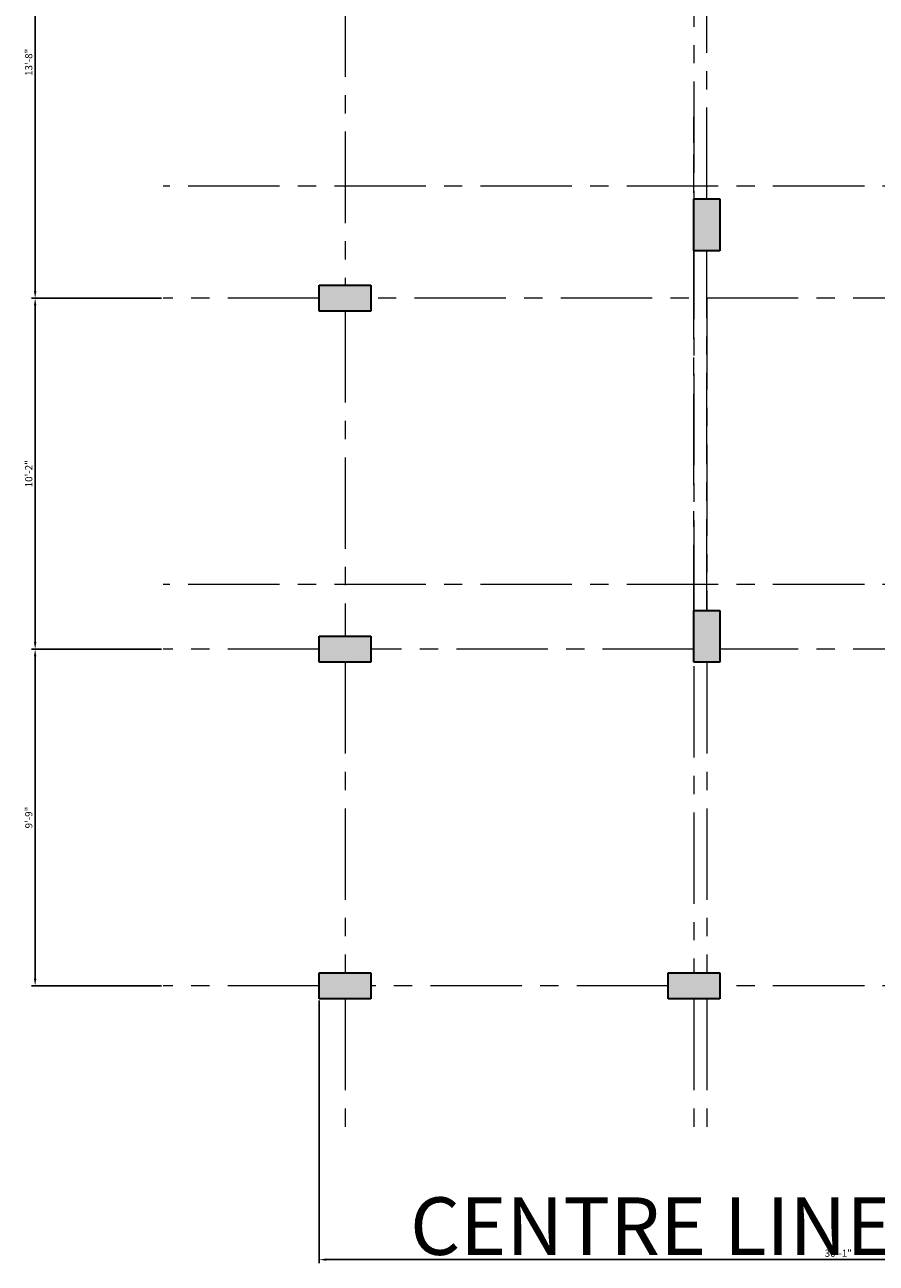
# Model space of a CAD drawing. Units: inches. Extents: x 2391 to 16591, y 7259 to 10239.
# Tile 22 of 27: x 3554 to 3850, y 9262 to 9693. Entities that reach past the tile are written whole.
import ezdxf

# ---------------------------------------------------------------- set-up
doc = ezdxf.new("R2010")
doc.units = ezdxf.units.IN
doc.linetypes.add('CENTER', pattern=[50.8, 31.75, -6.35, 6.35, -6.35])
for name, color, linetype, lineweight in [('A-ANNO-DIMS', 4, 'Continuous', 18), ('A-ANNO-TITL', 3, 'Continuous', 30), ('A-COLS', 3, 'Continuous', 35), ('A-COLS-PATT', 3, 'Continuous', 13), ('A-GRID', 1, 'CENTER', 13)]:
    doc.layers.add(name, color=color, linetype=linetype, lineweight=lineweight)
doc.styles.get("Standard").update_dxf_attribs({"font": 'arial.ttf'})
doc.dimstyles.new('ISO-25', dxfattribs={"dimtxt": 2.5, "dimasz": 2.5, "dimexe": 1.25, "dimexo": 0.625, "dimtad": 1, "dimdec": 0, "dimlunit": 3, "dimtxsty": 'Standard', "dimcen": 2.5, "dimadec": 0, "dimazin": 0, "dimtfac": 1, "dimtdec": 0, "dimtmove": 0, "dimatfit": 3, "dimfxl": 1, "dimarcsym": 0})

# ---------------------------------------------------------------- blocks, each defined once
blk = doc.blocks.new('*D102')
at = {"layer": 'A-ANNO-DIMS', "color": 0, "lineweight": -2, "transparency": 16777216}
for p, q in [((3656.26, 9353.63), (3656.26, 9262.37)), ((4017.01, 9353.63), (4017.01, 9262.37)), ((3658.76, 9263.62), (4014.51, 9263.62))]:
    blk.add_line(p, q, dxfattribs=at)
at = {"layer": 'A-ANNO-DIMS', "color": 0, "transparency": 16777216}
for points in [[(3658.76, 9264.03), (3658.76, 9263.2), (3656.26, 9263.62)], [(4014.51, 9264.03), (4014.51, 9263.2), (4017.01, 9263.62)]]:
    blk.add_solid(points, dxfattribs=at)
at = {"layer": 'Defpoints', "color": 0, "transparency": 16777216}
for p in [(3656.26, 9354.26), (4017.01, 9354.26), (4017.01, 9263.62)]:
    blk.add_point(p, dxfattribs=at)
at = {"layer": 'A-ANNO-DIMS', "color": 0, "transparency": 16777216, "insert": (3836.64, 9265.52), "char_height": 2.5, "attachment_point": 5}
blk.add_mtext('30\'-1"', dxfattribs=at)
blk = doc.blocks.new('*D107')
at = {"layer": 'A-ANNO-DIMS', "color": 0, "lineweight": -2, "transparency": 16777216}
for p, q in [((3601.45, 9475.76), (3556.32, 9475.76)), ((3557.57, 9361.26), (3557.57, 9473.26)), ((3601.45, 9358.76), (3556.32, 9358.76))]:
    blk.add_line(p, q, dxfattribs=at)
at = {"layer": 'A-ANNO-DIMS', "color": 0, "transparency": 16777216}
for points in [[(3557.15, 9473.26), (3557.99, 9473.26), (3557.57, 9475.76)], [(3557.15, 9361.26), (3557.99, 9361.26), (3557.57, 9358.76)]]:
    blk.add_solid(points, dxfattribs=at)
at = {"layer": 'Defpoints', "color": 0, "transparency": 16777216}
for p in [(3557.57, 9475.76), (3602.07, 9475.76), (3602.07, 9358.76)]:
    blk.add_point(p, dxfattribs=at)
at = {"layer": 'A-ANNO-DIMS', "color": 0, "transparency": 16777216, "insert": (3555.67, 9417.26), "char_height": 2.5, "attachment_point": 5, "rotation": 90}
blk.add_mtext('9\'-9"', dxfattribs=at)
blk = doc.blocks.new('*D108')
at = {"layer": 'A-ANNO-DIMS', "color": 0, "lineweight": -2, "transparency": 16777216}
for p, q in [((3601.45, 9597.76), (3556.32, 9597.76)), ((3557.57, 9478.26), (3557.57, 9595.26)), ((3601.45, 9475.76), (3556.32, 9475.76))]:
    blk.add_line(p, q, dxfattribs=at)
at = {"layer": 'A-ANNO-DIMS', "color": 0, "transparency": 16777216}
for points in [[(3557.15, 9595.26), (3557.99, 9595.26), (3557.57, 9597.76)], [(3557.15, 9478.26), (3557.99, 9478.26), (3557.57, 9475.76)]]:
    blk.add_solid(points, dxfattribs=at)
at = {"layer": 'Defpoints', "color": 0, "transparency": 16777216}
for p in [(3557.57, 9597.76), (3602.07, 9597.76), (3602.07, 9475.76)]:
    blk.add_point(p, dxfattribs=at)
at = {"layer": 'A-ANNO-DIMS', "color": 0, "transparency": 16777216, "insert": (3555.67, 9536.76), "char_height": 2.5, "attachment_point": 5, "rotation": 90}
blk.add_mtext('10\'-2"', dxfattribs=at)
blk = doc.blocks.new('*D109')
at = {"layer": 'A-ANNO-DIMS', "color": 0, "lineweight": -2, "transparency": 16777216}
for p, q in [((3601.45, 9761.76), (3556.32, 9761.76)), ((3557.57, 9600.26), (3557.57, 9759.26)), ((3601.45, 9597.76), (3556.32, 9597.76))]:
    blk.add_line(p, q, dxfattribs=at)
at = {"layer": 'A-ANNO-DIMS', "color": 0, "transparency": 16777216}
for points in [[(3557.15, 9759.26), (3557.99, 9759.26), (3557.57, 9761.76)], [(3557.15, 9600.26), (3557.99, 9600.26), (3557.57, 9597.76)]]:
    blk.add_solid(points, dxfattribs=at)
at = {"layer": 'Defpoints', "color": 0, "transparency": 16777216}
for p in [(3557.57, 9761.76), (3602.07, 9761.76), (3602.07, 9597.76)]:
    blk.add_point(p, dxfattribs=at)
at = {"layer": 'A-ANNO-DIMS', "color": 0, "transparency": 16777216, "insert": (3555.67, 9679.76), "char_height": 2.5, "attachment_point": 5, "rotation": 90}
blk.add_mtext('13\'-8"', dxfattribs=at)

msp = doc.modelspace()

# ---------------------------------------------------------------- hatches: boundary and pattern name
at = {"layer": 'A-COLS-PATT'}
h = msp.add_hatch(color=256, dxfattribs=at)
h.dxf.hatch_style = 1
h.paths.add_polyline_path([(3674.26, 9993.26), (3674.26, 10002.26), (3656.26, 10002.26), (3656.26, 9993.26)])
h.paths.add_polyline_path([(3777.51, 10002.26), (3777.51, 9993.26), (3795.51, 9993.26), (3795.51, 10002.26)])
h.paths.add_polyline_path([(3896.51, 10002.26), (3896.51, 9993.26), (3914.51, 9993.26), (3914.51, 10002.26)])
h.paths.add_polyline_path([(3999.01, 10002.26), (3999.01, 9993.26), (4017.01, 9993.26), (4017.01, 10002.26)])
h.paths.add_polyline_path([(4017.01, 9860.76), (4017.01, 9869.76), (3999.01, 9869.76), (3999.01, 9860.76)])
h.paths.add_polyline_path([(3914.51, 9860.76), (3914.51, 9869.76), (3896.51, 9869.76), (3896.51, 9860.76)])
h.paths.add_polyline_path([(3777.51, 9885.26), (3777.51, 9876.26), (3795.51, 9876.26), (3795.51, 9885.26)])
h.paths.add_polyline_path([(3674.26, 9876.26), (3674.26, 9885.26), (3656.26, 9885.26), (3656.26, 9876.26)])
h.paths.add_polyline_path([(3656.26, 9766.26), (3656.26, 9757.26), (3674.26, 9757.26), (3674.26, 9766.26)])
h.paths.add_polyline_path([(3786.51, 9759.76), (3795.51, 9759.76), (3795.51, 9777.76), (3786.51, 9777.76)])
h.paths.add_polyline_path([(3914.51, 9721.26), (3914.51, 9730.26), (3896.51, 9730.26), (3896.51, 9721.26)])
h.paths.add_polyline_path([(3999.01, 9730.26), (3999.01, 9721.26), (4017.01, 9721.26), (4017.01, 9730.26)])
h.paths.add_polyline_path([(4017.01, 9632.26), (4017.01, 9641.26), (3999.01, 9641.26), (3999.01, 9632.26)])
h.paths.add_polyline_path([(3914.51, 9632.26), (3914.51, 9641.26), (3896.51, 9641.26), (3896.51, 9632.26)])
h.paths.add_polyline_path([(3795.51, 9632.26), (3786.51, 9632.26), (3786.51, 9614.26), (3795.51, 9614.26)])
h.paths.add_polyline_path([(3656.26, 9602.26), (3656.26, 9593.26), (3674.26, 9593.26), (3674.26, 9602.26)])
h.paths.add_polyline_path([(3674.26, 9471.26), (3674.26, 9480.26), (3656.26, 9480.26), (3656.26, 9471.26)])
h.paths.add_polyline_path([(3795.51, 9489.26), (3786.51, 9489.26), (3786.51, 9471.26), (3795.51, 9471.26)])
h.paths.add_polyline_path([(3896.51, 9502.76), (3896.51, 9493.76), (3914.51, 9493.76), (3914.51, 9502.76)])
h.paths.add_polyline_path([(3999.01, 9502.76), (3999.01, 9493.76), (4017.01, 9493.76), (4017.01, 9502.76)])
h.paths.add_polyline_path([(4017.01, 9354.26), (4017.01, 9363.26), (3999.01, 9363.26), (3999.01, 9354.26)])
h.paths.add_polyline_path([(3914.51, 9354.26), (3914.51, 9363.26), (3896.51, 9363.26), (3896.51, 9354.26)])
h.paths.add_polyline_path([(3795.51, 9354.26), (3795.51, 9363.26), (3777.51, 9363.26), (3777.51, 9354.26)])
h.paths.add_polyline_path([(3674.26, 9354.26), (3674.26, 9363.26), (3656.26, 9363.26), (3656.26, 9354.26)])

# ---------------------------------------------------------------- linework, layer by layer
at = {"layer": 'A-COLS'}
for p, q in [((3786.51, 9614.26), (3786.51, 9632.26)), ((3786.51, 9632.26), (3795.51, 9632.26)), ((3795.51, 9632.26), (3795.51, 9614.26)), ((3795.51, 9614.26), (3786.51, 9614.26)), ((3656.26, 9602.26), (3674.26, 9602.26)), ((3656.26, 9593.26), (3656.26, 9602.26)), ((3674.26, 9602.26), (3674.26, 9593.26)), ((3674.26, 9593.26), (3656.26, 9593.26)), ((3786.51, 9471.26), (3786.51, 9489.26)), ((3786.51, 9489.26), (3795.51, 9489.26)), ((3795.51, 9489.26), (3795.51, 9471.26)), ((3656.26, 9480.26), (3674.26, 9480.26)), ((3656.26, 9471.26), (3656.26, 9480.26)), ((3674.26, 9480.26), (3674.26, 9471.26)), ((3674.26, 9471.26), (3656.26, 9471.26)), ((3795.51, 9471.26), (3786.51, 9471.26)), ((3656.26, 9363.26), (3674.26, 9363.26)), ((3656.26, 9354.26), (3656.26, 9363.26)), ((3674.26, 9363.26), (3674.26, 9354.26)), ((3777.51, 9363.26), (3795.51, 9363.26)), ((3777.51, 9354.26), (3777.51, 9363.26)), ((3795.51, 9363.26), (3795.51, 9354.26)), ((3674.26, 9354.26), (3656.26, 9354.26)), ((3795.51, 9354.26), (3777.51, 9354.26))]:
    msp.add_line(p, q, dxfattribs=at)
at = {"layer": 'A-GRID'}
for p, q in [((3786.51, 9876.26), (3786.51, 9363.26)), ((3791.01, 9632.26), (3791.01, 9759.76)), ((3665.26, 9757.26), (3665.26, 9602.26)), ((3786.51, 9651.76), (3786.51, 9660.76)), ((3786.51, 9532.76), (3786.51, 9647.76)), ((3896.51, 9636.76), (3602.07, 9636.76)), ((3791.01, 9489.26), (3791.01, 9614.26)), ((3656.26, 9597.76), (3602.07, 9597.76)), ((4076.77, 9597.76), (3674.26, 9597.76)), ((3791.01, 9597.76), (3791.01, 9489.26)), ((3665.26, 9593.26), (3665.26, 9480.26)), ((3786.51, 9480.26), (3786.51, 9523.76)), ((3896.51, 9498.26), (3602.07, 9498.26)), ((3656.26, 9475.76), (3602.07, 9475.76)), ((3786.51, 9475.76), (3674.26, 9475.76)), ((4076.77, 9475.76), (3795.51, 9475.76)), ((3665.26, 9471.26), (3665.26, 9363.26)), ((3791.01, 9471.26), (3791.01, 9363.26)), ((3656.26, 9358.76), (3602.07, 9358.76)), ((3777.51, 9358.76), (3674.26, 9358.76)), ((3896.51, 9358.76), (3795.51, 9358.76)), ((3665.26, 9354.26), (3665.26, 9308.12)), ((3786.51, 9354.26), (3786.51, 9308.12)), ((3791.01, 9354.26), (3791.01, 9308.12))]:
    msp.add_line(p, q, dxfattribs=at)

# ---------------------------------------------------------------- texts
at = {"layer": 'A-ANNO-TITL', "insert": (3687.85, 9285.26), "char_height": 20, "attachment_point": 1}
msp.add_mtext_dynamic_manual_height_columns('CENTRE LINE DIAGRAM', width=529.6372, gutter_width=12.5, heights=[0], dxfattribs=at)

# ---------------------------------------------------------------- dimensions: what is measured, and where the dimension line sits
at = {"layer": 'A-ANNO-DIMS'}
for base, p1, p2, picture, middle in [((3557.57, 9761.76), (3602.07, 9597.76), (3602.07, 9761.76), '*D109', (3555.67, 9679.76)), ((3557.57, 9597.76), (3602.07, 9475.76), (3602.07, 9597.76), '*D108', (3555.67, 9536.76)), ((3557.57, 9475.76), (3602.07, 9358.76), (3602.07, 9475.76), '*D107', (3555.67, 9417.26))]:
    dim = msp.add_linear_dim(base=base, p1=p1, p2=p2, angle=90, dimstyle='ISO-25', override={"dimdec": 1, "dimlfac": 1, "dimrnd": 0, "dimzin": 1, "dimdsep": 46, "dimlunit": 4, "dimfrac": 2}, dxfattribs=at)
    dim.commit()
    dim.dimension.update_dxf_attribs({"geometry": picture, "text_midpoint": middle})
dim = msp.add_linear_dim(base=(4017.01174, 9263.615693), p1=(3656.26174, 9354.257617), p2=(4017.01174, 9354.257617), dimstyle='ISO-25', override={"dimdec": 1, "dimlfac": 1, "dimrnd": 0, "dimzin": 1, "dimdsep": 46, "dimlunit": 4, "dimfrac": 2}, dxfattribs=at)
dim.commit()
dim.dimension.update_dxf_attribs({"geometry": '*D102', "text_midpoint": (3836.63674, 9265.51797813)})

doc.saveas('drawing.dxf')
